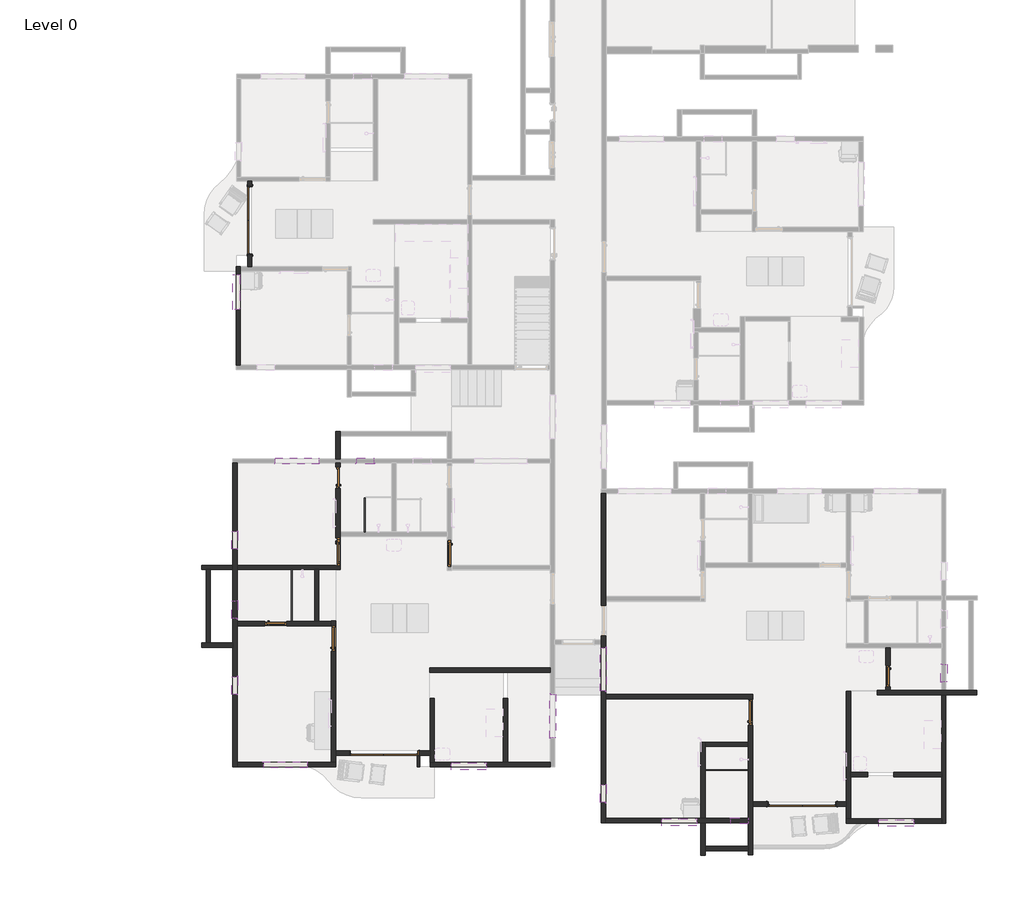
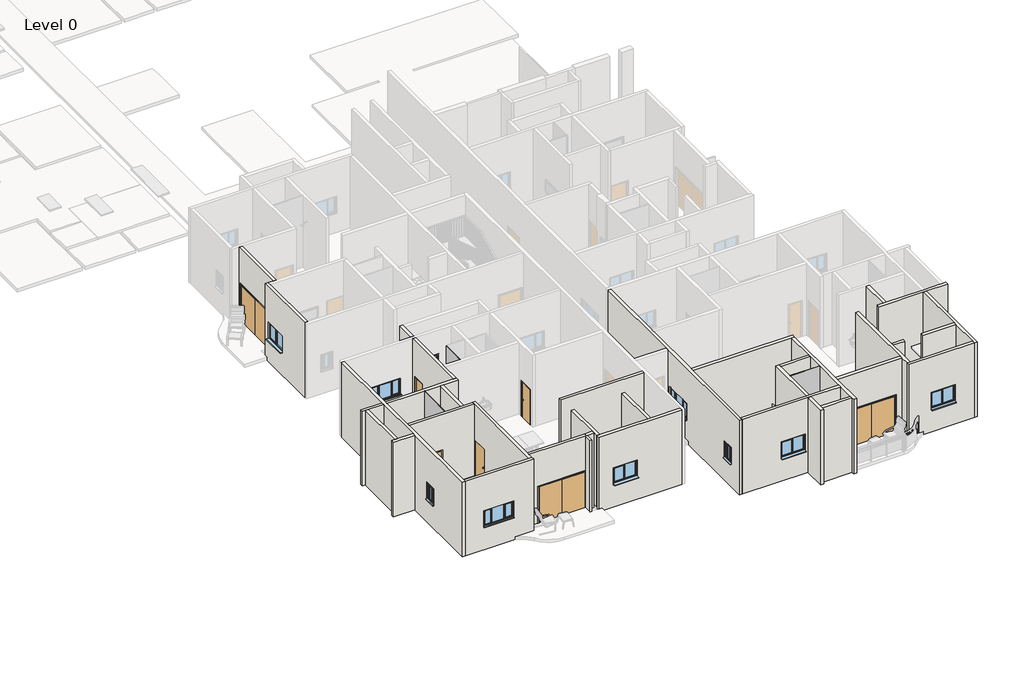
# One storey, part 1 of 14: 33 walls, 15 windows, 11 doors, 3 plates.
"""IFC4 building model written with IfcOpenShell, lengths in millimetres."""

from ifc_helpers import new_model, si_unit, frame, origin, origin_with_axes, place, context, project, spatial, polyline, outline, extrude, faceted_brep, transform, mapped, element, save
from components import doors_concept_intdbl_8_5090a96f, doors_concept_intdbl_8_9aa9adea, doors_extsgl_flush_d2_fac1298c, doors_extsgl_flush_d2_5e0ff3e2, doors_extsgl_flush_d3_352cde1d, doors_extsgl_flush_d3_ba5ff989, system_panel_glazed_095a6893, system_panel_glazed_e61de5c1, system_panel_glazed_61de1ab3, windows_concept_plain_dbl_4_d1e2e333, windows_sgl_plain_2_be143095, windows_tpl_variable_casement_2_47b04551, windows_tpl_variable_casement_5_ffad3fa3

model = new_model("IFC4")

# Units and contexts
model_context = context("Model", 3, world=origin())
ifc_project = project(units=[si_unit("LENGTHUNIT", "METRE", prefix="MILLI")], contexts=[model_context])

# Site, building, storey
site = spatial("IfcSite", under=ifc_project)
building = spatial("IfcBuilding", under=site)
storey = spatial("IfcBuildingStorey", under=building, Name="Level 0", Elevation=0.0)

# Doors
placement = place(None, origin())
doors_concept_intdbl_8_shape = doors_concept_intdbl_8_5090a96f(model_context)
element("IfcDoor", 1, ObjectType="Doors_Concept_IntDbl : 8'", at=placement, inside=storey, context=model_context, shape_type="MappedRepresentation", body=[
    mapped(doors_concept_intdbl_8_shape, transform((-12926.9935991, 10552.0590683, 0.0), x_axis=(-1.0, 0.0, 0.0), y_axis=(0.0, -1.0, 0.0), z_axis=(0.0, 0.0, 1.0))),
])
element("IfcDoor", 2, ObjectType="Doors_Concept_IntDbl : 8'", at=placement, inside=storey, context=model_context, shape_type="MappedRepresentation", body=[
    mapped(doors_concept_intdbl_8_shape, transform((-32279.6800447, 31010.4541094, 0.0), x_axis=(0.0, 1.0, 0.0), y_axis=(-1.0, 0.0, 0.0), z_axis=(0.0, 0.0, 1.0))),
])
doors_concept_intdbl_8_2_shape = doors_concept_intdbl_8_9aa9adea(model_context)
element("IfcDoor", 3, ObjectType="Doors_Concept_IntDbl : 8'", at=placement, inside=storey, context=model_context, shape_type="MappedRepresentation", body=[
    mapped(doors_concept_intdbl_8_2_shape, transform((-27581.0864125, 12335.6794818, 0.0), x_axis=(1.0, 0.0, 0.0), y_axis=(0.0, 1.0, 0.0), z_axis=(0.0, 0.0, 1.0))),
])
doors_extsgl_flush_d2_shape = doors_extsgl_flush_d2_fac1298c(model_context)
element("IfcDoor", 4, ObjectType="Doors_ExtSgl_Flush : D2", at=placement, inside=storey, context=model_context, shape_type="MappedRepresentation", body=[
    mapped(doors_extsgl_flush_d2_shape, transform((-29345.4063508, 16355.2294818, 0.0), x_axis=(0.0, 1.0, 0.0), y_axis=(-1.0, 0.0, 0.0), z_axis=(0.0, 0.0, 1.0))),
])
element("IfcDoor", 5, ObjectType="Doors_ExtSgl_Flush : D2", at=placement, inside=storey, context=model_context, shape_type="MappedRepresentation", body=[
    mapped(doors_extsgl_flush_d2_shape, transform((-25283.1553928, 19330.1762656, 0.0), x_axis=(0.0, -1.0, 0.0), y_axis=(1.0, 0.0, 0.0), z_axis=(0.0, 0.0, 1.0))),
])
element("IfcDoor", 6, ObjectType="Doors_ExtSgl_Flush : D2", at=placement, inside=storey, context=model_context, shape_type="MappedRepresentation", body=[
    mapped(doors_extsgl_flush_d2_shape, transform((-14739.2433343, 13771.5090683, 0.0), x_axis=(0.0, 1.0, 0.0), y_axis=(-1.0, 0.0, 0.0), z_axis=(0.0, 0.0, 1.0))),
])
doors_extsgl_flush_d2_2_shape = doors_extsgl_flush_d2_5e0ff3e2(model_context)
element("IfcDoor", 7, ObjectType="Doors_ExtSgl_Flush : D2", at=placement, inside=storey, context=model_context, shape_type="MappedRepresentation", body=[
    mapped(doors_extsgl_flush_d2_2_shape, transform((-29183.2280604, 19354.4580104, 0.0), x_axis=(0.0, -1.0, 0.0), y_axis=(1.0, 0.0, 0.0), z_axis=(0.0, 0.0, 1.0))),
])
element("IfcDoor", 8, ObjectType="Doors_ExtSgl_Flush : D2", at=placement, inside=storey, context=model_context, shape_type="MappedRepresentation", body=[
    mapped(doors_extsgl_flush_d2_2_shape, transform((-29183.2280604, 19416.0981245, 0.0), x_axis=(0.0, -1.0, 0.0), y_axis=(1.0, 0.0, 0.0), z_axis=(0.0, 0.0, 1.0))),
])
doors_extsgl_flush_d3_shape = doors_extsgl_flush_d3_352cde1d(model_context)
element("IfcDoor", 9, ObjectType="Doors_ExtSgl_Flush : D3", at=placement, inside=storey, context=model_context, shape_type="MappedRepresentation", body=[
    mapped(doors_extsgl_flush_d3_shape, transform((-31367.210195, 16877.7111792, 0.0), x_axis=(1.0, 0.0, 0.0), y_axis=(0.0, 1.0, 0.0), z_axis=(0.0, 0.0, 1.0))),
])
element("IfcDoor", 10, ObjectType="Doors_ExtSgl_Flush : D3", at=placement, inside=storey, context=model_context, shape_type="MappedRepresentation", body=[
    mapped(doors_extsgl_flush_d3_shape, transform((-9919.5953327, 15036.3736639, 0.0), x_axis=(0.0, -1.0, 0.0), y_axis=(1.0, 0.0, 0.0), z_axis=(0.0, 0.0, 1.0))),
])
doors_extsgl_flush_d3_2_shape = doors_extsgl_flush_d3_ba5ff989(model_context)
element("IfcDoor", 11, ObjectType="Doors_ExtSgl_Flush : D3", at=placement, inside=storey, context=model_context, shape_type="MappedRepresentation", body=[
    mapped(doors_extsgl_flush_d3_2_shape, transform((-29183.2280604, 21985.5411882, 0.0), x_axis=(0.0, 1.0, 0.0), y_axis=(-1.0, 0.0, 0.0), z_axis=(0.0, 0.0, 1.0))),
])

# Plates
system_panel_glazed_shape = system_panel_glazed_095a6893(model_context)
element("IfcPlate", 12, ObjectType="System Panel : Glazed", at=placement, inside=storey, context=model_context, shape_type="MappedRepresentation", body=[
    mapped(system_panel_glazed_shape, transform((-28213.4677419, 20677.4411882, 0.0), x_axis=(0.0, 1.0, 0.0), y_axis=(-1.0, 0.0, 0.0), z_axis=(0.0, 0.0, 1.0))),
])
system_panel_glazed_2_shape = system_panel_glazed_e61de5c1(model_context)
element("IfcPlate", 13, ObjectType="System Panel : Glazed", at=placement, inside=storey, context=model_context, shape_type="MappedRepresentation", body=[
    mapped(system_panel_glazed_2_shape, transform((-30848.9632392, 17860.1356661, 0.0), x_axis=(0.0, -1.0, 0.0), y_axis=(1.0, 0.0, 0.0), z_axis=(0.0, 0.0, 1.0))),
])
system_panel_glazed_3_shape = system_panel_glazed_61de1ab3(model_context)
element("IfcPlate", 14, ObjectType="System Panel : Glazed", at=placement, inside=storey, context=model_context, shape_type="MappedRepresentation", body=[
    mapped(system_panel_glazed_3_shape, transform((-15569.9354685, 11705.8999087, 0.0), x_axis=(1.0, 0.0, 0.0), y_axis=(0.0, 1.0, 0.0), z_axis=(0.0, 0.0, 1.0))),
])

# Walls
element("IfcWall", 15, ObjectType="W1", at=placement, inside=storey, context=model_context, shape_type="Brep", body=[
    faceted_brep([(-8043.7419991, 14375.9736639, 0.0), (-8043.7419991, 11663.0633156, 0.0), (-8043.7419991, 11510.6633156, 0.0), (-8043.7419991, 10026.1220639, 0.0), (-8043.7419991, 9873.7220639, 0.0), (-8043.7419991, 9873.7220639, 4000.0), (-8043.7419991, 10026.1220639, 4000.0), (-8043.7419991, 11510.6633156, 4000.0), (-8043.7419991, 11663.0633156, 4000.0), (-8043.7419991, 14375.9736639, 4000.0), (-7891.3419991, 14375.9736639, 0.0), (-7891.3419991, 14375.9736639, 4000.0), (-7891.3419991, 9873.7220639, 4000.0), (-7891.3419991, 9873.7220639, 0.0)], [[[0, 1, 2, 3, 4, 5, 6, 7, 8, 9]], [[10, 11, 12, 13]], [[4, 3, 2, 1, 0, 10, 13]], [[9, 8, 7, 6, 5, 12, 11]], [[5, 4, 13, 12]], [[0, 9, 11, 10]]]),
])
element("IfcWall", 16, ObjectType="W1", at=placement, inside=storey, context=model_context, shape_type="Brep", body=[
    faceted_brep([(-8043.7419991, 10026.1220639, 0.0), (-11225.1935991, 10026.1220639, 0.0), (-11377.5935991, 10026.1220639, 0.0), (-11377.5935991, 10026.1220639, 4000.0), (-11225.1935991, 10026.1220639, 4000.0), (-8043.7419991, 10026.1220639, 4000.0), (-9024.8677991, 10026.1220639, 2110.0), (-10244.0677991, 10026.1220639, 2110.0), (-10244.0677991, 10026.1220639, 1200.0), (-9024.8677991, 10026.1220639, 1200.0), (-8043.7419991, 9873.7220639, 0.0), (-8043.7419991, 9873.7220639, 4000.0), (-11377.5935991, 9873.7220639, 4000.0), (-11377.5935991, 9873.7220639, 0.0), (-9024.8677991, 9873.7220639, 2110.0), (-9024.8677991, 9873.7220639, 1200.0), (-10244.0677991, 9873.7220639, 1200.0), (-10244.0677991, 9873.7220639, 2110.0)], [[[0, 1, 2, 3, 4, 5], [6, 7, 8, 9]], [[10, 11, 12, 13], [14, 15, 16, 17]], [[2, 1, 0, 10, 13]], [[5, 4, 3, 12, 11]], [[0, 5, 11, 10]], [[3, 2, 13, 12]], [[15, 14, 6, 9]], [[16, 15, 9, 8]], [[17, 16, 8, 7]], [[14, 17, 7, 6]]]),
])
element("IfcWall", 17, ObjectType="W1", at=placement, inside=storey, context=model_context, shape_type="Brep", body=[
    faceted_brep([(-11225.1935991, 10026.1220639, 0.0), (-11225.1935991, 14509.3236639, 0.0), (-11225.1935991, 14509.3236639, 4000.0), (-11225.1935991, 10026.1220639, 4000.0), (-11377.5935991, 10026.1220639, 0.0), (-11377.5935991, 10026.1220639, 4000.0), (-11377.5935991, 10475.8590683, 4000.0), (-11377.5935991, 10628.2590683, 4000.0), (-11377.5935991, 14509.3236639, 4000.0), (-11377.5935991, 14509.3236639, 0.0), (-11377.5935991, 10628.2590683, 0.0), (-11377.5935991, 10475.8590683, 0.0)], [[[0, 1, 2, 3]], [[4, 5, 6, 7, 8, 9, 10, 11]], [[1, 0, 4, 11, 10, 9]], [[2, 1, 9, 8]], [[3, 2, 8, 7, 6, 5]], [[0, 3, 5, 4]]]),
])
element("IfcWall", 18, ObjectType="W1", at=placement, inside=storey, context=model_context, shape_type="Brep", body=[
    faceted_brep([(-10297.9919991, 14375.9736639, 0.0), (-8043.7419991, 14375.9736639, 0.0), (-7891.3419991, 14375.9736639, 0.0), (-6805.4919991, 14375.9736639, 0.0), (-6805.4919991, 14375.9736639, 4000.0), (-7891.3419991, 14375.9736639, 4000.0), (-8043.7419991, 14375.9736639, 4000.0), (-10297.9919991, 14375.9736639, 4000.0), (-10297.9919991, 14528.3736639, 0.0), (-10297.9919991, 14528.3736639, 4000.0), (-9995.7953327, 14528.3736639, 4000.0), (-9843.3953327, 14528.3736639, 4000.0), (-8039.9933343, 14528.3736639, 4000.0), (-7887.5933343, 14528.3736639, 4000.0), (-7089.3473173, 14528.3736639, 4000.0), (-6936.9473173, 14528.3736639, 4000.0), (-6805.4919991, 14528.3736639, 4000.0), (-6805.4919991, 14528.3736639, 0.0), (-6936.9473173, 14528.3736639, 0.0), (-7089.3473173, 14528.3736639, 0.0), (-7887.5933343, 14528.3736639, 0.0), (-8039.9933343, 14528.3736639, 0.0), (-9843.3953327, 14528.3736639, 0.0), (-9995.7953327, 14528.3736639, 0.0)], [[[0, 1, 2, 3, 4, 5, 6, 7]], [[8, 9, 10, 11, 12, 13, 14, 15, 16, 17, 18, 19, 20, 21, 22, 23]], [[3, 2, 1, 0, 8, 23, 22, 21, 20, 19, 18, 17]], [[4, 3, 17, 16]], [[7, 6, 5, 4, 16, 15, 14, 13, 12, 11, 10, 9]], [[0, 7, 9, 8]]]),
])
element("IfcWall", 19, ObjectType="W1", at=placement, inside=storey, context=model_context, shape_type="Brep", body=[
    faceted_brep([(-19965.3949343, 21442.5122683, 0.0), (-19965.3949343, 17512.8762397, 0.0), (-19965.3949343, 17512.8762397, 2110.0), (-19965.3949343, 16446.0762397, 2110.0), (-19965.3949343, 16446.0762397, 0.0), (-19965.3949343, 16301.243411, 0.0), (-19965.3949343, 16148.843411, 0.0), (-19965.3949343, 9898.1106683, 0.0), (-19965.3949343, 9898.1106683, 4000.0), (-19965.3949343, 16148.843411, 4000.0), (-19965.3949343, 16301.243411, 4000.0), (-19965.3949343, 21442.5122683, 4000.0), (-19965.3949343, 10609.3106683, 2110.0), (-19965.3949343, 10609.3106683, 1200.0), (-19965.3949343, 11218.9106683, 1200.0), (-19965.3949343, 11218.9106683, 2110.0), (-19965.3949343, 14509.3770397, 2110.0), (-19965.3949343, 14509.3770397, 1200.0), (-19965.3949343, 16033.3770397, 1200.0), (-19965.3949343, 16033.3770397, 2110.0), (-19812.9949343, 17512.8762397, 2110.0), (-19812.9949343, 17512.8762397, 0.0), (-19812.9949343, 17670.5106683, 0.0), (-19812.9949343, 17822.9106683, 0.0), (-19812.9949343, 21442.5122683, 0.0), (-19812.9949343, 21442.5122683, 4000.0), (-19812.9949343, 17822.9106683, 4000.0), (-19812.9949343, 17670.5106683, 4000.0), (-19812.9949343, 14393.9106683, 4000.0), (-19812.9949343, 14241.5106683, 4000.0), (-19812.9949343, 10050.5106683, 4000.0), (-19812.9949343, 9898.1106683, 4000.0), (-19812.9949343, 9898.1106683, 0.0), (-19812.9949343, 10050.5106683, 0.0), (-19812.9949343, 14241.5106683, 0.0), (-19812.9949343, 14393.9106683, 0.0), (-19812.9949343, 16446.0762397, 0.0), (-19812.9949343, 16446.0762397, 2110.0), (-19812.9949343, 10609.3106683, 2110.0), (-19812.9949343, 11218.9106683, 2110.0), (-19812.9949343, 11218.9106683, 1200.0), (-19812.9949343, 10609.3106683, 1200.0), (-19812.9949343, 14509.3770397, 2110.0), (-19812.9949343, 16033.3770397, 2110.0), (-19812.9949343, 16033.3770397, 1200.0), (-19812.9949343, 14509.3770397, 1200.0)], [[[0, 1, 2, 3, 4, 5, 6, 7, 8, 9, 10, 11], [12, 13, 14, 15], [16, 17, 18, 19]], [[20, 21, 22, 23, 24, 25, 26, 27, 28, 29, 30, 31, 32, 33, 34, 35, 36, 37], [38, 39, 40, 41], [42, 43, 44, 45]], [[24, 23, 22, 21, 1, 0]], [[36, 35, 34, 33, 32, 7, 6, 5, 4]], [[11, 10, 9, 8, 31, 30, 29, 28, 27, 26, 25]], [[0, 11, 25, 24]], [[8, 7, 32, 31]], [[4, 3, 37, 36]], [[2, 1, 21, 20]], [[3, 2, 20, 37]], [[13, 12, 38, 41]], [[14, 13, 41, 40]], [[15, 14, 40, 39]], [[12, 15, 39, 38]], [[17, 16, 42, 45]], [[18, 17, 45, 44]], [[19, 18, 44, 43]], [[16, 19, 43, 42]]]),
])
element("IfcWall", 20, ObjectType="W1", at=placement, inside=storey, context=model_context, shape_type="Brep", body=[
    faceted_brep([(-19812.9949343, 14241.5106683, 0.0), (-14815.4433343, 14241.5106683, 0.0), (-14663.0433343, 14241.5106683, 0.0), (-14663.0433343, 14241.5106683, 4000.0), (-14815.4433343, 14241.5106683, 4000.0), (-19812.9949343, 14241.5106683, 4000.0), (-19812.9949343, 14393.9106683, 0.0), (-19812.9949343, 14393.9106683, 4000.0), (-14663.0433343, 14393.9106683, 4000.0), (-14663.0433343, 14393.9106683, 0.0)], [[[0, 1, 2, 3, 4, 5]], [[6, 7, 8, 9]], [[2, 1, 0, 6, 9]], [[5, 4, 3, 8, 7]], [[0, 5, 7, 6]], [[3, 2, 9, 8]]]),
])
element("IfcWall", 21, ObjectType="W1", at=placement, inside=storey, context=model_context, shape_type="Brep", body=[
    faceted_brep([(-14815.4433343, 8767.7090683, 0.0), (-14815.4433343, 8767.7090683, 4000.0), (-14815.4433343, 8911.8999087, 4000.0), (-14815.4433343, 9064.2999087, 4000.0), (-14815.4433343, 9898.1106683, 4000.0), (-14815.4433343, 10050.5106683, 4000.0), (-14815.4433343, 12569.4999087, 4000.0), (-14815.4433343, 12721.8999087, 4000.0), (-14815.4433343, 14241.5106683, 4000.0), (-14815.4433343, 14241.5106683, 0.0), (-14815.4433343, 14228.7090683, 0.0), (-14815.4433343, 14228.7090683, 2110.0), (-14815.4433343, 13314.3090683, 2110.0), (-14815.4433343, 13314.3090683, 0.0), (-14815.4433343, 12721.8999087, 0.0), (-14815.4433343, 12569.4999087, 0.0), (-14815.4433343, 10050.5106683, 0.0), (-14815.4433343, 9898.1106683, 0.0), (-14815.4433343, 9064.2999087, 0.0), (-14815.4433343, 8911.8999087, 0.0), (-14663.0433343, 8767.7090683, 4000.0), (-14663.0433343, 8767.7090683, 0.0), (-14663.0433343, 10475.8590683, 0.0), (-14663.0433343, 10628.2590683, 0.0), (-14663.0433343, 13314.3090683, 0.0), (-14663.0433343, 13314.3090683, 2110.0), (-14663.0433343, 14228.7090683, 2110.0), (-14663.0433343, 14228.7090683, 0.0), (-14663.0433343, 14241.5106683, 0.0), (-14663.0433343, 14241.5106683, 4000.0), (-14663.0433343, 10628.2590683, 4000.0), (-14663.0433343, 10475.8590683, 4000.0)], [[[0, 1, 2, 3, 4, 5, 6, 7, 8, 9, 10, 11, 12, 13, 14, 15, 16, 17, 18, 19]], [[20, 21, 22, 23, 24, 25, 26, 27, 28, 29, 30, 31]], [[21, 0, 19, 18, 17, 16, 15, 14, 13, 24, 23, 22]], [[9, 28, 27, 10]], [[1, 0, 21, 20]], [[8, 7, 6, 5, 4, 3, 2, 1, 20, 31, 30, 29]], [[9, 8, 29, 28]], [[12, 25, 24, 13]], [[26, 11, 10, 27]], [[25, 12, 11, 26]]]),
])
element("IfcWall", 22, ObjectType="W1", at=placement, inside=storey, context=model_context, shape_type="Brep", body=[
    faceted_brep([(-14815.4433343, 9898.1106683, 0.0), (-14815.4433343, 9898.1106683, 1828.9328), (-15425.0433343, 9898.1106683, 1828.9328), (-15425.0433343, 9898.1106683, 2738.9328), (-14815.4433343, 9898.1106683, 2738.9328), (-14815.4433343, 9898.1106683, 4000.0), (-16324.4276027, 9898.1106683, 4000.0), (-16476.8276027, 9898.1106683, 4000.0), (-19812.9949343, 9898.1106683, 4000.0), (-19812.9949343, 9898.1106683, 0.0), (-16476.8276027, 9898.1106683, 0.0), (-16324.4276027, 9898.1106683, 0.0), (-16618.8433343, 9898.1106683, 2110.0), (-16618.8433343, 9898.1106683, 1200.0), (-17838.0433343, 9898.1106683, 1200.0), (-17838.0433343, 9898.1106683, 2110.0), (-15425.0433343, 10050.5106683, 1828.9328), (-14815.4433343, 10050.5106683, 1828.9328), (-14815.4433343, 10050.5106683, 0.0), (-16324.4276027, 10050.5106683, 0.0), (-16476.8276027, 10050.5106683, 0.0), (-19812.9949343, 10050.5106683, 0.0), (-19812.9949343, 10050.5106683, 4000.0), (-16476.8276027, 10050.5106683, 4000.0), (-16324.4276027, 10050.5106683, 4000.0), (-14815.4433343, 10050.5106683, 4000.0), (-14815.4433343, 10050.5106683, 2738.9328), (-15425.0433343, 10050.5106683, 2738.9328), (-16618.8433343, 10050.5106683, 2110.0), (-17838.0433343, 10050.5106683, 2110.0), (-17838.0433343, 10050.5106683, 1200.0), (-16618.8433343, 10050.5106683, 1200.0)], [[[0, 1, 2, 3, 4, 5, 6, 7, 8, 9, 10, 11], [12, 13, 14, 15]], [[16, 17, 18, 19, 20, 21, 22, 23, 24, 25, 26, 27], [28, 29, 30, 31]], [[0, 11, 10, 9, 21, 20, 19, 18]], [[8, 7, 6, 5, 25, 24, 23, 22]], [[9, 8, 22, 21]], [[26, 25, 5, 4]], [[18, 17, 1, 0]], [[13, 12, 28, 31]], [[14, 13, 31, 30]], [[15, 14, 30, 29]], [[12, 15, 29, 28]], [[2, 1, 17, 16]], [[3, 2, 16, 27]], [[4, 3, 27, 26]]]),
])
element("IfcWall", 23, ObjectType="W1", at=placement, inside=storey, context=model_context, shape_type="Brep", body=[
    faceted_brep([(-16476.8276027, 8759.4999087, 0.0), (-16476.8276027, 8759.4999087, 4000.0), (-16476.8276027, 9898.1106683, 4000.0), (-16476.8276027, 9898.1106683, 0.0), (-16324.4276027, 8759.4999087, 4000.0), (-16324.4276027, 8759.4999087, 0.0), (-16324.4276027, 8911.8999087, 0.0), (-16324.4276027, 9064.2999087, 0.0), (-16324.4276027, 9898.1106683, 0.0), (-16324.4276027, 9898.1106683, 4000.0), (-16324.4276027, 9064.2999087, 4000.0), (-16324.4276027, 8911.8999087, 4000.0)], [[[0, 1, 2, 3]], [[4, 5, 6, 7, 8, 9, 10, 11]], [[5, 0, 3, 8, 7, 6]], [[1, 0, 5, 4]], [[1, 4, 11, 10, 9, 2]], [[3, 2, 9, 8]]]),
    faceted_brep([(-16476.8276027, 12721.8999087, 4000.0), (-16476.8276027, 12721.8999087, 0.0), (-16476.8276027, 10050.5106683, 0.0), (-16476.8276027, 10050.5106683, 4000.0), (-16324.4276027, 12721.8999087, 0.0), (-16324.4276027, 12721.8999087, 4000.0), (-16324.4276027, 12569.4999087, 4000.0), (-16324.4276027, 10050.5106683, 4000.0), (-16324.4276027, 10050.5106683, 0.0), (-16324.4276027, 12569.4999087, 0.0)], [[[0, 1, 2, 3]], [[4, 5, 6, 7, 8, 9]], [[1, 4, 9, 8, 2]], [[5, 0, 3, 7, 6]], [[1, 0, 5, 4]], [[3, 2, 8, 7]]]),
])
element("IfcWall", 24, ObjectType="W1", at=placement, inside=storey, context=model_context, shape_type="SweptSolid", body=[
    extrude(outline(polyline([(-14815.4433343, 12569.4999087), (-16324.4276027, 12569.4999087), (-16324.4276027, 12721.8999087), (-14815.4433343, 12721.8999087), (-14815.4433343, 12569.4999087)])), origin_with_axes(), (0.0, 0.0, 1.0), 4000.0),
])
element("IfcWall", 25, ObjectType="W1", at=placement, inside=storey, context=model_context, shape_type="SweptSolid", body=[
    extrude(outline(polyline([(14655.3736639, 2110.0), (14655.3736639, 0.0), (14528.3736639, 0.0), (14528.3736639, 4000.0), (16023.4530766, 4000.0), (16023.4530766, 0.0), (15417.3736639, 0.0), (15417.3736639, 2110.0), (14655.3736639, 2110.0)])), frame((-9995.7953327, 0.0, 0.0), z_axis=(1.0, 0.0, 0.0), x_axis=(0.0, 1.0, 0.0)), (0.0, 0.0, 1.0), 152.4),
])
element("IfcWall", 26, ObjectType="W1", at=placement, inside=storey, context=model_context, shape_type="SweptSolid", body=[
    extrude(outline(polyline([(4000.0, -11377.5935991), (4000.0, -14663.0433343), (0.0, -14663.0433343), (0.0, -14146.1935991), (2110.0, -14146.1935991), (2110.0, -11707.7935991), (0.0, -11707.7935991), (0.0, -11377.5935991), (4000.0, -11377.5935991)])), frame((0.0, 10475.8590683, 0.0), z_axis=(0.0, 1.0, 0.0), x_axis=(0.0, 0.0, 1.0)), (0.0, 0.0, 1.0), 152.4),
])
element("IfcWall", 27, ObjectType="W1", at=placement, inside=storey, context=model_context, shape_type="Brep", body=[
    faceted_brep([(-21744.3547508, 12011.8294818, 0.0), (-23242.9901022, 12011.8294818, 0.0), (-23395.3901022, 12011.8294818, 0.0), (-25808.4563508, 12011.8294818, 0.0), (-25960.8563508, 12011.8294818, 0.0), (-25960.8563508, 12011.8294818, 4000.0), (-25808.4563508, 12011.8294818, 4000.0), (-23395.3901022, 12011.8294818, 4000.0), (-23242.9901022, 12011.8294818, 4000.0), (-21744.3547508, 12011.8294818, 4000.0), (-23998.7240265, 12011.8294818, 2110.0), (-25217.9240265, 12011.8294818, 2110.0), (-25217.9240265, 12011.8294818, 1200.0), (-23998.7240265, 12011.8294818, 1200.0), (-21744.3547508, 11859.4294818, 0.0), (-21744.3547508, 11859.4294818, 4000.0), (-25960.8563508, 11859.4294818, 4000.0), (-25960.8563508, 11859.4294818, 0.0), (-23998.7240265, 11859.4294818, 2110.0), (-23998.7240265, 11859.4294818, 1200.0), (-25217.9240265, 11859.4294818, 1200.0), (-25217.9240265, 11859.4294818, 2110.0)], [[[0, 1, 2, 3, 4, 5, 6, 7, 8, 9], [10, 11, 12, 13]], [[14, 15, 16, 17], [18, 19, 20, 21]], [[4, 3, 2, 1, 0, 14, 17]], [[9, 8, 7, 6, 5, 16, 15]], [[0, 9, 15, 14]], [[5, 4, 17, 16]], [[19, 18, 10, 13]], [[20, 19, 13, 12]], [[21, 20, 12, 11]], [[18, 21, 11, 10]]]),
])
element("IfcWall", 28, ObjectType="W1", at=placement, inside=storey, context=model_context, shape_type="Brep", body=[
    faceted_brep([(-32875.9555508, 22500.1601529, 0.0), (-32875.9555508, 18918.7601529, 0.0), (-32875.9555508, 18766.3601529, 0.0), (-32875.9555508, 16191.7518714, 0.0), (-32875.9555508, 16039.3518714, 0.0), (-32875.9555508, 11859.4294818, 0.0), (-32875.9555508, 11859.4294818, 4000.0), (-32875.9555508, 16039.3518714, 4000.0), (-32875.9555508, 16191.7518714, 4000.0), (-32875.9555508, 18766.3601529, 4000.0), (-32875.9555508, 18918.7601529, 4000.0), (-32875.9555508, 22500.1601529, 4000.0), (-32875.9555508, 14401.1095792, 2110.0), (-32875.9555508, 14401.1095792, 1200.0), (-32875.9555508, 15010.7095792, 1200.0), (-32875.9555508, 15010.7095792, 2110.0), (-32875.9555508, 17055.5111792, 2738.9328), (-32875.9555508, 17055.5111792, 1828.9328), (-32875.9555508, 17665.1111792, 1828.9328), (-32875.9555508, 17665.1111792, 2738.9328), (-32875.9555508, 19493.9111792, 2110.0), (-32875.9555508, 19493.9111792, 1200.0), (-32875.9555508, 20103.5111792, 1200.0), (-32875.9555508, 20103.5111792, 2110.0), (-32723.5555508, 22500.1601529, 0.0), (-32723.5555508, 22500.1601529, 4000.0), (-32723.5555508, 18918.7601529, 4000.0), (-32723.5555508, 18766.3601529, 4000.0), (-32723.5555508, 16953.9111792, 4000.0), (-32723.5555508, 16801.5111792, 4000.0), (-32723.5555508, 12011.8294818, 4000.0), (-32723.5555508, 11859.4294818, 4000.0), (-32723.5555508, 11859.4294818, 0.0), (-32723.5555508, 12011.8294818, 0.0), (-32723.5555508, 16801.5111792, 0.0), (-32723.5555508, 16953.9111792, 0.0), (-32723.5555508, 18766.3601529, 0.0), (-32723.5555508, 18918.7601529, 0.0), (-32723.5555508, 14401.1095792, 2110.0), (-32723.5555508, 15010.7095792, 2110.0), (-32723.5555508, 15010.7095792, 1200.0), (-32723.5555508, 14401.1095792, 1200.0), (-32723.5555508, 17055.5111792, 2738.9328), (-32723.5555508, 17665.1111792, 2738.9328), (-32723.5555508, 17665.1111792, 1828.9328), (-32723.5555508, 17055.5111792, 1828.9328), (-32723.5555508, 19493.9111792, 2110.0), (-32723.5555508, 20103.5111792, 2110.0), (-32723.5555508, 20103.5111792, 1200.0), (-32723.5555508, 19493.9111792, 1200.0)], [[[0, 1, 2, 3, 4, 5, 6, 7, 8, 9, 10, 11], [12, 13, 14, 15], [16, 17, 18, 19], [20, 21, 22, 23]], [[24, 25, 26, 27, 28, 29, 30, 31, 32, 33, 34, 35, 36, 37], [38, 39, 40, 41], [42, 43, 44, 45], [46, 47, 48, 49]], [[5, 4, 3, 2, 1, 0, 24, 37, 36, 35, 34, 33, 32]], [[11, 10, 9, 8, 7, 6, 31, 30, 29, 28, 27, 26, 25]], [[0, 11, 25, 24]], [[6, 5, 32, 31]], [[13, 12, 38, 41]], [[14, 13, 41, 40]], [[15, 14, 40, 39]], [[12, 15, 39, 38]], [[17, 16, 42, 45]], [[18, 17, 45, 44]], [[19, 18, 44, 43]], [[16, 19, 43, 42]], [[21, 20, 46, 49]], [[22, 21, 49, 48]], [[23, 22, 48, 47]], [[20, 23, 47, 46]]]),
])
element("IfcWall", 29, ObjectType="W1", at=placement, inside=storey, context=model_context, shape_type="Brep", body=[
    faceted_brep([(-32723.5555508, 11859.4294818, 0.0), (-29269.2063508, 11859.4294818, 0.0), (-29269.2063508, 11859.4294818, 4000.0), (-32723.5555508, 11859.4294818, 4000.0), (-30272.6079508, 11859.4294818, 2110.0), (-30272.6079508, 11859.4294818, 1200.0), (-31796.6079508, 11859.4294818, 1200.0), (-31796.6079508, 11859.4294818, 2110.0), (-32723.5555508, 12011.8294818, 0.0), (-32723.5555508, 12011.8294818, 4000.0), (-29421.6063508, 12011.8294818, 4000.0), (-29269.2063508, 12011.8294818, 4000.0), (-29269.2063508, 12011.8294818, 0.0), (-29421.6063508, 12011.8294818, 0.0), (-30272.6079508, 12011.8294818, 2110.0), (-31796.6079508, 12011.8294818, 2110.0), (-31796.6079508, 12011.8294818, 1200.0), (-30272.6079508, 12011.8294818, 1200.0)], [[[0, 1, 2, 3], [4, 5, 6, 7]], [[8, 9, 10, 11, 12, 13], [14, 15, 16, 17]], [[1, 0, 8, 13, 12]], [[3, 2, 11, 10, 9]], [[0, 3, 9, 8]], [[2, 1, 12, 11]], [[5, 4, 14, 17]], [[6, 5, 17, 16]], [[7, 6, 16, 15]], [[4, 7, 15, 14]]]),
])
element("IfcWall", 30, ObjectType="W1", at=placement, inside=storey, context=model_context, shape_type="Brep", body=[
    faceted_brep([(-29269.2063508, 16812.4294818, 2110.0), (-29269.2063508, 16812.4294818, 0.0), (-29269.2063508, 16964.8294818, 0.0), (-29269.2063508, 16964.8294818, 4000.0), (-29269.2063508, 12411.8794818, 4000.0), (-29269.2063508, 12259.4794818, 4000.0), (-29269.2063508, 12011.8294818, 4000.0), (-29269.2063508, 12011.8294818, 0.0), (-29269.2063508, 12259.4794818, 0.0), (-29269.2063508, 12411.8794818, 0.0), (-29269.2063508, 15898.0294818, 0.0), (-29269.2063508, 15898.0294818, 2110.0), (-29421.6063508, 16964.8294818, 0.0), (-29421.6063508, 16953.9111792, 0.0), (-29421.6063508, 16812.4294818, 0.0), (-29421.6063508, 16812.4294818, 2110.0), (-29421.6063508, 15898.0294818, 2110.0), (-29421.6063508, 15898.0294818, 0.0), (-29421.6063508, 12011.8294818, 0.0), (-29421.6063508, 12011.8294818, 4000.0), (-29421.6063508, 16801.5111792, 4000.0), (-29421.6063508, 16953.9111792, 4000.0), (-29421.6063508, 16964.8294818, 4000.0)], [[[0, 1, 2, 3, 4, 5, 6, 7, 8, 9, 10, 11]], [[12, 13, 14, 15, 16, 17, 18, 19, 20, 21, 22]], [[2, 1, 14, 13, 12]], [[10, 9, 8, 7, 18, 17]], [[3, 2, 12, 22]], [[6, 5, 4, 3, 22, 21, 20, 19]], [[7, 6, 19, 18]], [[17, 16, 11, 10]], [[15, 14, 1, 0]], [[16, 15, 0, 11]]]),
])
element("IfcWall", 31, ObjectType="W1", at=placement, inside=storey, context=model_context, shape_type="Brep", body=[
    faceted_brep([(-30986.210195, 16801.5111792, 2110.0), (-30986.210195, 16801.5111792, 0.0), (-29421.6063508, 16801.5111792, 0.0), (-29421.6063508, 16801.5111792, 4000.0), (-32723.5555508, 16801.5111792, 4000.0), (-32723.5555508, 16801.5111792, 0.0), (-31748.210195, 16801.5111792, 0.0), (-31748.210195, 16801.5111792, 2110.0), (-29421.6063508, 16953.9111792, 0.0), (-29858.3632392, 16953.9111792, 0.0), (-30010.7632392, 16953.9111792, 0.0), (-30986.210195, 16953.9111792, 0.0), (-30986.210195, 16953.9111792, 2110.0), (-31748.210195, 16953.9111792, 2110.0), (-31748.210195, 16953.9111792, 0.0), (-32723.5555508, 16953.9111792, 0.0), (-32723.5555508, 16953.9111792, 4000.0), (-30010.7632392, 16953.9111792, 4000.0), (-29858.3632392, 16953.9111792, 4000.0), (-29421.6063508, 16953.9111792, 4000.0), (-29421.6063508, 16812.4294818, 0.0)], [[[0, 1, 2, 3, 4, 5, 6, 7]], [[8, 9, 10, 11, 12, 13, 14, 15, 16, 17, 18, 19]], [[6, 5, 15, 14]], [[2, 1, 11, 10, 9, 8, 20]], [[4, 3, 19, 18, 17, 16]], [[5, 4, 16, 15]], [[3, 2, 20, 8, 19]], [[14, 13, 7, 6]], [[12, 11, 1, 0]], [[13, 12, 0, 7]]]),
])
element("IfcWall", 32, ObjectType="W1", at=placement, inside=storey, context=model_context, shape_type="Brep", body=[
    faceted_brep([(-33964.7780604, 18766.3601529, 4000.0), (-33964.7780604, 18766.3601529, 0.0), (-33812.3780604, 18766.3601529, 0.0), (-33659.9780604, 18766.3601529, 0.0), (-32875.9555508, 18766.3601529, 0.0), (-32875.9555508, 18766.3601529, 4000.0), (-33659.9780604, 18766.3601529, 4000.0), (-33812.3780604, 18766.3601529, 4000.0), (-33964.7780604, 18918.7601529, 0.0), (-33964.7780604, 18918.7601529, 4000.0), (-32875.9555508, 18918.7601529, 4000.0), (-32875.9555508, 18918.7601529, 0.0)], [[[0, 1, 2, 3, 4, 5, 6, 7]], [[8, 9, 10, 11]], [[1, 8, 11, 4, 3, 2]], [[9, 0, 7, 6, 5, 10]], [[1, 0, 9, 8]], [[5, 4, 11, 10]]]),
    faceted_brep([(-29107.0280604, 18766.3601529, 0.0), (-29107.0280604, 18766.3601529, 4000.0), (-29858.3632392, 18766.3601529, 4000.0), (-30010.7632392, 18766.3601529, 4000.0), (-32723.5555508, 18766.3601529, 4000.0), (-32723.5555508, 18766.3601529, 0.0), (-30010.7632392, 18766.3601529, 0.0), (-29858.3632392, 18766.3601529, 0.0), (-29107.0280604, 18918.7601529, 4000.0), (-29107.0280604, 18918.7601529, 2110.0), (-29259.4280604, 18918.7601529, 2110.0), (-29259.4280604, 18918.7601529, 0.0), (-32723.5555508, 18918.7601529, 0.0), (-32723.5555508, 18918.7601529, 4000.0), (-29259.4280604, 18918.7601529, 4000.0), (-29107.0280604, 18897.2580104, 0.0), (-29259.4280604, 18897.2580104, 0.0), (-29107.0280604, 18897.2580104, 2110.0), (-29259.4280604, 18897.2580104, 2110.0)], [[[0, 1, 2, 3, 4, 5, 6, 7]], [[8, 9, 10, 11, 12, 13, 14]], [[15, 0, 7, 6, 5, 12, 11, 16]], [[1, 8, 14, 13, 4, 3, 2]], [[5, 4, 13, 12]], [[1, 0, 15, 17, 9, 8]], [[18, 16, 11, 10]], [[16, 18, 17, 15]], [[17, 18, 10, 9]]]),
])
element("IfcWall", 33, ObjectType="W1", at=placement, inside=storey, context=model_context, shape_type="SweptSolid", body=[
    extrude(outline(polyline([(-30010.7632392, 16953.9111792), (-30010.7632392, 18766.3601529), (-29858.3632392, 18766.3601529), (-29858.3632392, 16953.9111792), (-30010.7632392, 16953.9111792)])), origin_with_axes(), (0.0, 0.0, 1.0), 4000.0),
])
element("IfcWall", 34, ObjectType="W1", at=placement, inside=storey, context=model_context, shape_type="Brep", body=[
    faceted_brep([(-29259.4280604, 18918.7601529, 2110.0), (-29259.4280604, 18918.7601529, 4000.0), (-29259.4280604, 22500.1601529, 4000.0), (-29259.4280604, 22500.1601529, 0.0), (-29259.4280604, 22366.5411882, 0.0), (-29259.4280604, 22366.5411882, 2110.0), (-29259.4280604, 21604.5411882, 2110.0), (-29259.4280604, 21604.5411882, 0.0), (-29259.4280604, 19873.2981245, 0.0), (-29259.4280604, 19873.2981245, 2110.0), (-29107.0280604, 18918.7601529, 4000.0), (-29107.0280604, 18918.7601529, 2110.0), (-29107.0280604, 19873.2981245, 2110.0), (-29107.0280604, 19873.2981245, 0.0), (-29107.0280604, 19928.1411882, 0.0), (-29107.0280604, 20080.5411882, 0.0), (-29107.0280604, 21604.5411882, 0.0), (-29107.0280604, 21604.5411882, 2110.0), (-29107.0280604, 22366.5411882, 2110.0), (-29107.0280604, 22366.5411882, 0.0), (-29107.0280604, 22500.1601529, 0.0), (-29107.0280604, 22500.1601529, 4000.0), (-29107.0280604, 20080.5411882, 4000.0), (-29107.0280604, 19928.1411882, 4000.0)], [[[0, 1, 2, 3, 4, 5, 6, 7, 8, 9]], [[10, 11, 12, 13, 14, 15, 16, 17, 18, 19, 20, 21, 22, 23]], [[13, 8, 7, 16, 15, 14]], [[19, 4, 3, 20]], [[1, 10, 23, 22, 21, 2]], [[3, 2, 21, 20]], [[10, 1, 0, 11]], [[11, 0, 9, 12]], [[12, 9, 8, 13]], [[7, 6, 17, 16]], [[5, 4, 19, 18]], [[6, 5, 18, 17]]]),
    faceted_brep([(-29259.4280604, 23611.1411882, 4000.0), (-29259.4280604, 23611.1411882, 0.0), (-29259.4280604, 22652.5601529, 0.0), (-29259.4280604, 22652.5601529, 4000.0), (-29107.0280604, 23611.1411882, 0.0), (-29107.0280604, 23611.1411882, 4000.0), (-29107.0280604, 23458.7411882, 4000.0), (-29107.0280604, 22652.5601529, 4000.0), (-29107.0280604, 22652.5601529, 0.0), (-29107.0280604, 23458.7411882, 0.0)], [[[0, 1, 2, 3]], [[4, 5, 6, 7, 8, 9]], [[1, 4, 9, 8, 2]], [[5, 0, 3, 7, 6]], [[3, 2, 8, 7]], [[1, 0, 5, 4]]]),
])
element("IfcWall", 35, ObjectType="W1", at=placement, inside=storey, context=model_context, shape_type="SweptSolid", body=[
    extrude(outline(polyline([(-21744.3547508, 15172.0304681), (-25975.6710986, 15172.0304681), (-25975.6710986, 15324.4304681), (-21744.3547508, 15324.4304681), (-21744.3547508, 15172.0304681)])), origin_with_axes(), (0.0, 0.0, 1.0), 4000.0),
])
element("IfcWall", 36, ObjectType="W1", at=placement, inside=storey, context=model_context, shape_type="Brep", body=[
    faceted_brep([(-25808.4563508, 12011.8294818, 0.0), (-25808.4563508, 14259.8310818, 0.0), (-25808.4563508, 14259.8310818, 4000.0), (-25808.4563508, 12011.8294818, 4000.0), (-25960.8563508, 12011.8294818, 0.0), (-25960.8563508, 12011.8294818, 4000.0), (-25960.8563508, 12256.9800791, 4000.0), (-25960.8563508, 12409.3800791, 4000.0), (-25960.8563508, 14259.8310818, 4000.0), (-25960.8563508, 14259.8310818, 0.0), (-25960.8563508, 12409.3800791, 0.0), (-25960.8563508, 12256.9800791, 0.0)], [[[0, 1, 2, 3]], [[4, 5, 6, 7, 8, 9, 10, 11]], [[1, 0, 4, 11, 10, 9]], [[2, 1, 9, 8]], [[3, 2, 8, 7, 6, 5]], [[0, 3, 5, 4]]]),
])
element("IfcWall", 37, ObjectType="W1", at=placement, inside=storey, context=model_context, shape_type="SweptSolid", body=[
    extrude(outline(polyline([(-23242.9901022, 14259.8310818), (-23242.9901022, 12011.8294818), (-23395.3901022, 12011.8294818), (-23395.3901022, 14259.8310818), (-23242.9901022, 14259.8310818)])), origin_with_axes(), (0.0, 0.0, 1.0), 4000.0),
])
element("IfcWall", 38, ObjectType="W1", at=placement, inside=storey, context=model_context, shape_type="Brep", body=[
    faceted_brep([(-25960.8563508, 12409.3800791, 0.0), (-26361.8864125, 12409.3800791, 0.0), (-26361.8864125, 12409.3800791, 4000.0), (-25960.8563508, 12409.3800791, 4000.0), (-25960.8563508, 12256.9800791, 0.0), (-25960.8563508, 12256.9800791, 4000.0), (-26316.1664125, 12256.9800791, 4000.0), (-26361.8864125, 12256.9800791, 4000.0), (-26361.8864125, 12256.9800791, 0.0), (-26316.1664125, 12256.9800791, 0.0), (-26361.8864125, 12259.4794818, 0.0), (-26361.8864125, 12259.4794818, 4000.0)], [[[0, 1, 2, 3]], [[4, 5, 6, 7, 8, 9]], [[1, 0, 4, 9, 8, 10]], [[2, 1, 10, 8, 7, 11]], [[3, 2, 11, 7, 6, 5]], [[0, 3, 5, 4]]]),
])
element("IfcWall", 39, ObjectType="W1", at=placement, inside=storey, context=model_context, shape_type="Brep", body=[
    faceted_brep([(-26361.8864125, 12259.4794818, 4000.0), (-26407.6064125, 12259.4794818, 4000.0), (-29269.2063508, 12259.4794818, 4000.0), (-29269.2063508, 12259.4794818, 0.0), (-28800.2864125, 12259.4794818, 0.0), (-28800.2864125, 12259.4794818, 2110.0), (-26361.8864125, 12259.4794818, 2110.0), (-29269.2063508, 12411.8794818, 4000.0), (-26361.8864125, 12411.8794818, 4000.0), (-26361.8864125, 12411.8794818, 2110.0), (-28800.2864125, 12411.8794818, 2110.0), (-28800.2864125, 12411.8794818, 0.0), (-29269.2063508, 12411.8794818, 0.0), (-26361.8864125, 12409.3800791, 4000.0)], [[[0, 1, 2, 3, 4, 5, 6]], [[7, 8, 9, 10, 11, 12]], [[3, 12, 11, 4]], [[8, 13, 0, 6, 9]], [[2, 1, 0, 13, 8, 7]], [[3, 2, 7, 12]], [[5, 10, 9, 6]], [[10, 5, 4, 11]]]),
])
element("IfcWall", 40, ObjectType="W1", at=placement, inside=storey, context=model_context, shape_type="Brep", body=[
    faceted_brep([(-32609.8800447, 25935.1270746, 0.0), (-32609.8800447, 29230.7770746, 0.0), (-32609.8800447, 29383.1770746, 0.0), (-32609.8800447, 29383.1770746, 4000.0), (-32609.8800447, 29230.7770746, 4000.0), (-32609.8800447, 25935.1270746, 4000.0), (-32609.8800447, 27884.5770746, 2110.0), (-32609.8800447, 29103.7770746, 2110.0), (-32609.8800447, 29103.7770746, 1200.0), (-32609.8800447, 27884.5770746, 1200.0), (-32762.2800447, 25935.1270746, 0.0), (-32762.2800447, 25935.1270746, 4000.0), (-32762.2800447, 29383.1770746, 4000.0), (-32762.2800447, 29383.1770746, 0.0), (-32762.2800447, 27884.5770746, 2110.0), (-32762.2800447, 27884.5770746, 1200.0), (-32762.2800447, 29103.7770746, 1200.0), (-32762.2800447, 29103.7770746, 2110.0)], [[[0, 1, 2, 3, 4, 5], [6, 7, 8, 9]], [[10, 11, 12, 13], [14, 15, 16, 17]], [[2, 1, 0, 10, 13]], [[5, 4, 3, 12, 11]], [[0, 5, 11, 10]], [[3, 2, 13, 12]], [[15, 14, 6, 9]], [[16, 15, 9, 8]], [[17, 16, 8, 7]], [[14, 17, 7, 6]]]),
])
element("IfcWall", 41, ObjectType="W1", at=placement, inside=storey, context=model_context, shape_type="SweptSolid", body=[
    extrude(outline(polyline([(29383.1770746, 4000.0), (32382.0541094, 4000.0), (32382.0541094, 0.0), (32229.6541094, 0.0), (32229.6541094, 2110.0), (29791.2541094, 2110.0), (29791.2541094, 0.0), (29383.1770746, 0.0), (29383.1770746, 4000.0)])), frame((-32355.8800447, 0.0, 0.0), z_axis=(1.0, 0.0, 0.0), x_axis=(0.0, 1.0, 0.0)), (0.0, 0.0, 1.0), 152.4),
])
element("IfcWall", 42, ObjectType="W1", at=placement, inside=storey, context=model_context, shape_type="Brep", body=[
    faceted_brep([(-32875.9555508, 16191.7518714, 0.0), (-33659.9780604, 16191.7518714, 0.0), (-33812.3780604, 16191.7518714, 0.0), (-33968.1555508, 16191.7518714, 0.0), (-33968.1555508, 16191.7518714, 4000.0), (-33812.3780604, 16191.7518714, 4000.0), (-33659.9780604, 16191.7518714, 4000.0), (-32875.9555508, 16191.7518714, 4000.0), (-32875.9555508, 16039.3518714, 0.0), (-32875.9555508, 16039.3518714, 4000.0), (-33968.1555508, 16039.3518714, 4000.0), (-33968.1555508, 16039.3518714, 0.0)], [[[0, 1, 2, 3, 4, 5, 6, 7]], [[8, 9, 10, 11]], [[3, 2, 1, 0, 8, 11]], [[4, 3, 11, 10]], [[7, 6, 5, 4, 10, 9]], [[0, 7, 9, 8]]]),
])
element("IfcWall", 43, ObjectType="W1", at=placement, inside=storey, context=model_context, shape_type="SweptSolid", body=[
    extrude(outline(polyline([(-9720.1419991, 11663.0633156), (-8043.7419991, 11663.0633156), (-8043.7419991, 11510.6633156), (-9720.1419991, 11510.6633156), (-9720.1419991, 11663.0633156)])), origin_with_axes(), (0.0, 0.0, 1.0), 4000.0),
])
element("IfcWall", 44, ObjectType="W1", at=placement, inside=storey, context=model_context, shape_type="SweptSolid", body=[
    extrude(outline(polyline([(-11218.7419991, 11663.0633156), (-10634.5419991, 11663.0633156), (-10634.5419991, 11510.6633156), (-11218.7419991, 11510.6633156), (-11218.7419991, 11663.0633156)])), origin_with_axes(), (0.0, 0.0, 1.0), 4000.0),
])
element("IfcWall", 45, ObjectType="W1", at=placement, inside=storey, context=model_context, shape_type="SweptSolid", body=[
    extrude(outline(polyline([(-33812.3780604, 16191.7518714), (-33812.3780604, 18766.3601529), (-33659.9780604, 18766.3601529), (-33659.9780604, 16191.7518714), (-33812.3780604, 16191.7518714)])), origin_with_axes(), (0.0, 0.0, 1.0), 4000.0),
])
element("IfcWall", 46, ObjectType="W1", at=placement, inside=storey, context=model_context, shape_type="SweptSolid", body=[
    extrude(outline(polyline([(-14815.4433343, 8911.8999087), (-16324.4276027, 8911.8999087), (-16324.4276027, 9064.2999087), (-14815.4433343, 9064.2999087), (-14815.4433343, 8911.8999087)])), origin_with_axes(), (0.0, 0.0, 1.0), 4000.0),
])
element("IfcWall", 47, ObjectType="W9", at=placement, inside=storey, context=model_context, shape_type="Brep", body=[
    faceted_brep([(-26407.6064125, 12259.4794818, 0.0), (-26407.6064125, 11859.4294818, 0.0), (-26407.6064125, 11859.4294818, 4000.0), (-26407.6064125, 12259.4794818, 4000.0), (-26316.1664125, 12256.9800791, 0.0), (-26316.1664125, 12256.9800791, 4000.0), (-26316.1664125, 11859.4294818, 4000.0), (-26316.1664125, 11859.4294818, 0.0), (-26361.8864125, 12259.4794818, 0.0), (-26361.8864125, 12256.9800791, 0.0), (-26361.8864125, 12256.9800791, 4000.0), (-26361.8864125, 12259.4794818, 4000.0), (-26361.8864125, 12256.9800791, 2110.0), (-26361.8864125, 12256.9800791, 1200.0)], [[[0, 1, 2, 3]], [[4, 5, 6, 7]], [[1, 0, 8, 9, 4, 7]], [[2, 1, 7, 6]], [[3, 2, 6, 5, 10, 11]], [[0, 3, 11, 8]], [[11, 10, 12, 13, 9, 8]], [[10, 5, 4, 9, 13, 12]]]),
])

# Windows
windows_concept_plain_dbl_4_shape = windows_concept_plain_dbl_4_d1e2e333(model_context)
element("IfcWindow", 48, ObjectType="Windows_Concept_Plain_Dbl : 4'", at=placement, inside=storey, context=model_context, shape_type="MappedRepresentation", body=[
    mapped(windows_concept_plain_dbl_4_shape, transform((-24893.3240265, 11944.0860497, 0.0), x_axis=(-1.0, 0.0, 0.0), y_axis=(0.0, -1.0, 0.0), z_axis=(0.0, 0.0, 1.0))),
])
element("IfcWindow", 49, ObjectType="Windows_Concept_Plain_Dbl : 4'", at=placement, inside=storey, context=model_context, shape_type="MappedRepresentation", body=[
    mapped(windows_concept_plain_dbl_4_shape, transform((-17513.4433343, 9982.7672362, 0.0), x_axis=(-1.0, 0.0, 0.0), y_axis=(0.0, -1.0, 0.0), z_axis=(0.0, 0.0, 1.0))),
])
element("IfcWindow", 50, ObjectType="Windows_Concept_Plain_Dbl : 4'", at=placement, inside=storey, context=model_context, shape_type="MappedRepresentation", body=[
    mapped(windows_concept_plain_dbl_4_shape, transform((-9919.4677991, 9958.3786317, 0.0), x_axis=(-1.0, 0.0, 0.0), y_axis=(0.0, -1.0, 0.0), z_axis=(0.0, 0.0, 1.0))),
])
element("IfcWindow", 51, ObjectType="Windows_Concept_Plain_Dbl : 4'", at=placement, inside=storey, context=model_context, shape_type="MappedRepresentation", body=[
    mapped(windows_concept_plain_dbl_4_shape, transform((-32677.6234769, 28779.1770746, 0.0), x_axis=(0.0, 1.0, 0.0), y_axis=(-1.0, 0.0, 0.0), z_axis=(0.0, 0.0, 1.0))),
])
windows_sgl_plain_2_shape = windows_sgl_plain_2_be143095(model_context)
element("IfcWindow", 52, ObjectType="Windows_Sgl_Plain : 2'", at=placement, inside=storey, context=model_context, shape_type="MappedRepresentation", body=[
    mapped(windows_sgl_plain_2_shape, transform((-32791.2989829, 17360.3111792, 628.9328), x_axis=(0.0, 1.0, 0.0), y_axis=(-1.0, 0.0, 0.0), z_axis=(0.0, 0.0, 1.0))),
])
element("IfcWindow", 53, ObjectType="Windows_Sgl_Plain : 2'", at=placement, inside=storey, context=model_context, shape_type="MappedRepresentation", body=[
    mapped(windows_sgl_plain_2_shape, transform((-28234.4090234, 22567.9035851, 628.9328), x_axis=(1.0, 0.0, 0.0), y_axis=(0.0, 1.0, 0.0), z_axis=(0.0, 0.0, 1.0))),
])
element("IfcWindow", 54, ObjectType="Windows_Sgl_Plain : 2'", at=placement, inside=storey, context=model_context, shape_type="MappedRepresentation", body=[
    mapped(windows_sgl_plain_2_shape, transform((-7972.2499021, 15137.9736639, 628.9328), x_axis=(0.0, -1.0, 0.0), y_axis=(1.0, 0.0, 0.0), z_axis=(0.0, 0.0, 1.0))),
])
element("IfcWindow", 55, ObjectType="Windows_Sgl_Plain : 2'", at=placement, inside=storey, context=model_context, shape_type="MappedRepresentation", body=[
    mapped(windows_sgl_plain_2_shape, transform((-15120.2433343, 9982.7672362, 628.9328), x_axis=(-1.0, 0.0, 0.0), y_axis=(0.0, -1.0, 0.0), z_axis=(0.0, 0.0, 1.0))),
])
windows_tpl_variable_casement_2_shape = windows_tpl_variable_casement_2_47b04551(model_context)
element("IfcWindow", 56, ObjectType="Windows_Tpl_Variable_Casement : 2'", at=placement, inside=storey, context=model_context, shape_type="MappedRepresentation", body=[
    mapped(windows_tpl_variable_casement_2_shape, transform((-32791.2989829, 14695.7095792, 0.0), x_axis=(0.0, 1.0, 0.0), y_axis=(-1.0, 0.0, 0.0), z_axis=(0.0, 0.0, 1.0))),
])
element("IfcWindow", 57, ObjectType="Windows_Tpl_Variable_Casement : 2'", at=placement, inside=storey, context=model_context, shape_type="MappedRepresentation", body=[
    mapped(windows_tpl_variable_casement_2_shape, transform((-32791.2989829, 19788.5111792, 0.0), x_axis=(0.0, 1.0, 0.0), y_axis=(-1.0, 0.0, 0.0), z_axis=(0.0, 0.0, 1.0))),
])
element("IfcWindow", 58, ObjectType="Windows_Tpl_Variable_Casement : 2'", at=placement, inside=storey, context=model_context, shape_type="MappedRepresentation", body=[
    mapped(windows_tpl_variable_casement_2_shape, transform((-19880.7383665, 10903.9106683, 0.0), x_axis=(0.0, 1.0, 0.0), y_axis=(-1.0, 0.0, 0.0), z_axis=(0.0, 0.0, 1.0))),
])
windows_tpl_variable_casement_5_shape = windows_tpl_variable_casement_5_ffad3fa3(model_context)
element("IfcWindow", 59, ObjectType="Windows_Tpl_Variable_Casement : 5'", at=placement, inside=storey, context=model_context, shape_type="MappedRepresentation", body=[
    mapped(windows_tpl_variable_casement_5_shape, transform((-31481.6079508, 11944.0860497, 0.0), x_axis=(-1.0, 0.0, 0.0), y_axis=(0.0, -1.0, 0.0), z_axis=(0.0, 0.0, 1.0))),
])
element("IfcWindow", 60, ObjectType="Windows_Tpl_Variable_Casement : 5'", at=placement, inside=storey, context=model_context, shape_type="MappedRepresentation", body=[
    mapped(windows_tpl_variable_casement_5_shape, transform((-30178.0322871, 22567.9035851, 0.0), x_axis=(1.0, 0.0, 0.0), y_axis=(0.0, 1.0, 0.0), z_axis=(0.0, 0.0, 1.0))),
])
element("IfcWindow", 61, ObjectType="Windows_Tpl_Variable_Casement : 5'", at=placement, inside=storey, context=model_context, shape_type="MappedRepresentation", body=[
    mapped(windows_tpl_variable_casement_5_shape, transform((-21676.6113186, 13188.2288681, 0.0), x_axis=(0.0, -1.0, 0.0), y_axis=(1.0, 0.0, 0.0), z_axis=(0.0, 0.0, 1.0))),
])
element("IfcWindow", 62, ObjectType="Windows_Tpl_Variable_Casement : 5'", at=placement, inside=storey, context=model_context, shape_type="MappedRepresentation", body=[
    mapped(windows_tpl_variable_casement_5_shape, transform((-19880.7383665, 15718.3770397, 0.0), x_axis=(0.0, 1.0, 0.0), y_axis=(-1.0, 0.0, 0.0), z_axis=(0.0, 0.0, 1.0))),
])

save(model, "model.ifc")

# Revit data of these elements
# Type "Doors_Concept_IntDbl : 8'"
#   Type Mark = "53"
#   Type Comments = "Internal Double"
#   Operation = "DoubleDoorSingleSwing"
#   Construction Type Id = "GSP4R"
#   Keynote = "L10"
#   Description = "Internal Double Door"
#   Analytic Construction = "1/8 in Pilkington single glazing"
#   Visual Light Transmittance = 0.9
#   Thickness = 32 mm
#   Solar Heat Gain Coefficient = 0.78
#   Rough Width = 2438.4 mm
#   Rough Height = 2110 mm
#   Height = 2110 mm
#   Width = 2438.4 mm
#   Heat Transfer Coefficient (U) = 3.6886 W/(m²·K)
#   Define Thermal Properties by = 1
#   Function = 1
#   Material Glass = Glass
#   Material Frame = Glass, Clear Glazing
#   Material Door = Glass
#   Material Architrave = Glass
#   Wall Closure = (empty or 0)
#   Assembly Code = ""
# Type "Doors_ExtSgl_Flush : D2"
#   Type Mark = "50"
#   Type Comments = "External Single"
#   Operation = "SingleSwingRight"
#   Construction Type Id = "MDOOR"
#   Keynote = "L20"
#   Analytic Construction = "Metal"
#   Wrap Layers (Int) from Ext = 177.5 mm
#   Wrap Layers (Ext) from Ext = 102.5 mm
#   Thickness = 44 mm
#   Rough Width = 914.4 mm
#   Rough Height = 2110 mm
#   O/A Frame Width = 64 mm
#   Heat Transfer Coefficient (U) = 3.7021 W/(m²·K)
#   Handle Z Distance = 1050 mm
#   FrameWidth = 42 mm
#   FrameOffset - External = 25 mm
#   FrameDepth = 89 mm
#   Door Panel Width = 811.4 mm
#   Door Panel Thickness = 44 mm
#   Door Panel Height = 2000 mm
#   Cill Thickness = 54.5 mm
#   Cill Projection = 30 mm
#   Handle X Distance = 75 mm
#   Height = 2110 mm
#   Structural Tolerance = 6.5 mm
#   Tolerance = 3 mm
#   Undercut = 4 mm
#   Width = 914.4 mm
#   Cill Extension = 25 mm
#   Cavity Closer Width = 50 mm
#   Cavity Closer Offset from Ext = 102.5 mm
#   Cavity Closer Depth = 85 mm
#   Vis - Ironmongery = yes
#   Vis - Cavity Closers = yes
#   Define Thermal Properties by = 1
#   Function = 1
#   Material Door = Door - Panel
#   Material Frame = Door - Frame/Mullion
#   Material Ironmongery = Door - Handle
#   Visual Light Transmittance = 0
#   Solar Heat Gain Coefficient = 0
#   Wall Closure = (empty or 0)
# Type "Doors_ExtSgl_Flush : D3"
#   Type Mark = "51"
#   Type Comments = "External Single"
#   Operation = "SingleSwingRight"
#   Construction Type Id = "MDOOR"
#   Keynote = "L20"
#   Analytic Construction = "Metal"
#   Wrap Layers (Int) from Ext = 177.5 mm
#   Wrap Layers (Ext) from Ext = 102.5 mm
#   Thickness = 44 mm
#   Rough Width = 762 mm
#   Rough Height = 2110 mm
#   O/A Frame Width = 64 mm
#   Heat Transfer Coefficient (U) = 3.7021 W/(m²·K)
#   Handle Z Distance = 1050 mm
#   FrameWidth = 42 mm
#   FrameOffset - External = 25 mm
#   FrameDepth = 89 mm
#   Door Panel Width = 659 mm
#   Door Panel Thickness = 44 mm
#   Door Panel Height = 2000 mm
#   Cill Thickness = 54.5 mm
#   Cill Projection = 30 mm
#   Handle X Distance = 75 mm
#   Height = 2110 mm
#   Structural Tolerance = 6.5 mm
#   Tolerance = 3 mm
#   Undercut = 4 mm
#   Width = 762 mm
#   Cill Extension = 25 mm
#   Cavity Closer Width = 50 mm
#   Cavity Closer Offset from Ext = 102.5 mm
#   Cavity Closer Depth = 85 mm
#   Vis - Ironmongery = yes
#   Vis - Cavity Closers = yes
#   Define Thermal Properties by = 1
#   Function = 1
#   Material Door = Door - Panel
#   Material Frame = Door - Frame/Mullion
#   Material Ironmongery = Door - Handle
#   Visual Light Transmittance = 0
#   Solar Heat Gain Coefficient = 0
#   Wall Closure = (empty or 0)
# Type "System Panel : Glazed"
#   Keynote = "H11"
#   Construction Type Id = "GSP4R"
#   Analytic Construction = "1/8 in Pilkington single glazing"
#   Visual Light Transmittance = 0.9
#   Solar Heat Gain Coefficient = 0.86
#   Heat Transfer Coefficient (U) = 6.7069 W/(m²·K)
#   Define Thermal Properties by = 1
# Type "W1"
#   Keynote = "F10"
#   Layers, outside or top first: 152.4 mm "Brick, Common" (function 1)
# Type "W9"
#   Keynote = "F10"
#   Layers, outside or top first: 91.44 mm "Brick, Common" (function 1)
# Type "Windows_Concept_Plain_Dbl : 4'"
#   Type Mark = "56"
#   Operation = "DoublePanelVertical"
#   Construction Type Id = "GSP4R"
#   Manufacturer = "Revit"
#   Keynote = "L10"
#   Analytic Construction = "1/8 in Pilkington single glazing"
#   Visual Light Transmittance = 0.9
#   Solar Heat Gain Coefficient = 0.78
#   Rough Width = 1219.2 mm
#   Rough Height = 910 mm
#   Height = 910 mm
#   Width = 1219.2 mm
#   Heat Transfer Coefficient (U) = 3.6886 W/(m²·K)
#   FrameOffset - External = 50 mm
#   Default Head Height = 2110 mm
#   Vis - Cavity Closers = yes
#   Define Thermal Properties by = 1
#   Material Trim = Window Frame
#   Material Glass = Glass
#   Material Frame = Window Frame
#   Wall Closure = (empty or 0)
# Type "Windows_Sgl_Plain : 2'"
#   Type Mark = "72"
#   Operation = "SinglePanel"
#   Construction Type Id = "SGL"
#   Manufacturer = "Revit"
#   Keynote = "L10"
#   Analytic Construction = "Large single-glazed windows"
#   Wrap Layers (Ext) from Ext = 102.5 mm
#   Wrap Layers (Int) from Ext = 177.5 mm
#   Window Board Projection = 25 mm
#   Window Board Extension = 25 mm
#   Visual Light Transmittance = 0.9
#   Solar Heat Gain Coefficient = 0.86
#   Rough Width = 609.6 mm
#   Rough Height = 910 mm
#   Height = 910 mm
#   Width = 609.6 mm
#   Heat Transfer Coefficient (U) = 5.5617 W/(m²·K)
#   Glazing Thickness = 24 mm
#   FrameOffset - External = 50 mm
#   Frame Depth = 65 mm
#   Default Head Height = 2110 mm
#   Cill Depth = 87.5 mm
#   Cavity Closer Width = 50 mm
#   Cavity Closer Offset from Ext = 102.5 mm
#   Cavity Closer Depth = 85 mm
#   Vis - Cavity Closers = yes
#   Define Thermal Properties by = 1
#   Material Trim = Window Frame
#   Material Glass = Glass
#   Material Frame = Window Frame
#   Wall Closure = (empty or 0)
# Type "Windows_Tpl_Variable_Casement : 2'"
#   Type Mark = "82"
#   Operation = "TriplePanelVertical"
#   Construction Type Id = "GSP4R"
#   Manufacturer = "Revit"
#   Keynote = "L10"
#   Analytic Construction = "1/8 in Pilkington single glazing"
#   Wrap Layers (Int) from Ext = 177.5 mm
#   Wrap Layers (Ext) from Ext = 102.5 mm
#   Window Board Projection = 25 mm
#   Window Board Extension = 25 mm
#   Visual Light Transmittance = 0.9
#   Solar Heat Gain Coefficient = 0.78
#   Rough Width = 609.6 mm
#   Rough Height = 910 mm
#   Height = 910 mm
#   Width = 609.6 mm
#   Heat Transfer Coefficient (U) = 3.6886 W/(m²·K)
#   Glazing Thickness = 24 mm
#   FrameOffset - External = 50 mm
#   Frame Depth = 65 mm
#   Default Head Height = 2110 mm
#   Cill Depth = 87.5 mm
#   Cavity Closer Width = 50 mm
#   Cavity Closer Offset from Ext = 102.5 mm
#   Cavity Closer Depth = 85 mm
#   Casement Width = 450 mm
#   Vis - Cavity Closers = yes
#   Define Thermal Properties by = 1
#   Material Trim = Window Frame
#   Material Glass = Glass
#   Material Frame = Window Frame
#   Wall Closure = (empty or 0)
# Type "Windows_Tpl_Variable_Casement : 5'"
#   Type Mark = "83"
#   Operation = "TriplePanelVertical"
#   Construction Type Id = "GSP4R"
#   Manufacturer = "Revit"
#   Keynote = "L10"
#   Analytic Construction = "1/8 in Pilkington single glazing"
#   Wrap Layers (Int) from Ext = 177.5 mm
#   Wrap Layers (Ext) from Ext = 102.5 mm
#   Window Board Projection = 25 mm
#   Window Board Extension = 25 mm
